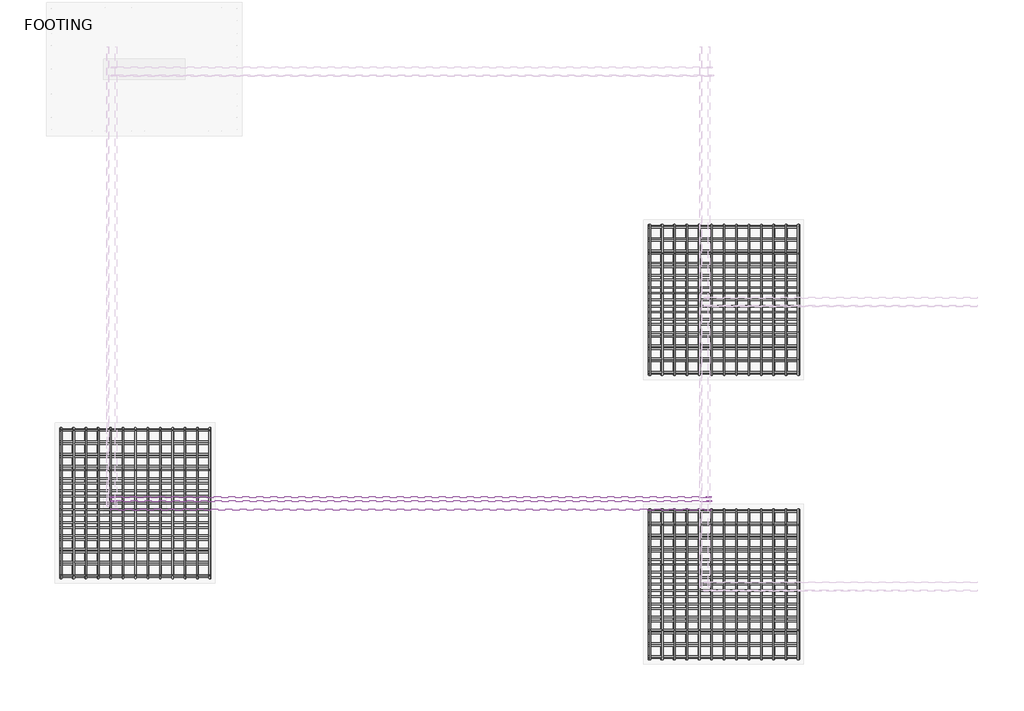
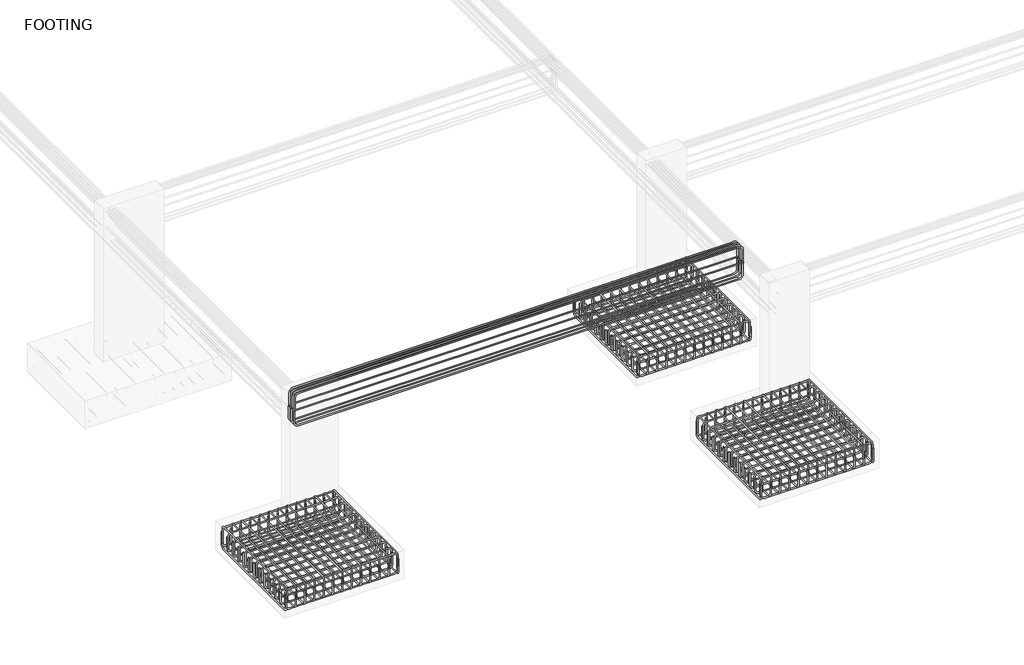
# One storey, part 2 of 12: 15 reinforcing bars.
"""IFC4 building model written with IfcOpenShell, lengths in millimetres."""

from ifc_helpers import new_model, si_unit, point, frame, origin, place, context, project, spatial, polyline, circle_curve, trimmed, segment, composite_curve, source, transform, mapped, element, save
from ifc_brep_helpers import swept_disk

model = new_model("IFC4")

# Units and contexts
model_context = context("Model", 3, world=origin())
ifc_project = project(units=[si_unit("LENGTHUNIT", "METRE", prefix="MILLI")], contexts=[model_context])

# Site, building, storey
site = spatial("IfcSite", under=ifc_project)
building = spatial("IfcBuilding", under=site)
storey = spatial("IfcBuildingStorey", under=building, Name="FOOTING", Elevation=-5638.8)

# Reinforcing bars
placement = place(None, origin())
reinforcing_bar_shape = source(origin(), model_context, "Body", "SolidModel", [
    swept_disk(composite_curve([segment(polyline([(-7583.1001665, -10857.5541655, -5788.8), (-7583.1001665, -10857.5541655, -5975.4)]), True, "CONTINUOUS"), segment(trimmed(circle_curve(frame((-7583.1001665, -10802.1041655, -5975.4), z_axis=(1.0, 0.0, 0.0), x_axis=(0.0, -55.44999999999891, 0.0)), 55.45), [point((-7583.1001665, -10857.5541655, -5975.4))], [point((-7583.1001665, -10802.1041655, -6030.85))], True, "CARTESIAN"), True, "CONTINUOUS"), segment(polyline([(-7583.1001665, -10802.1041655, -6030.85), (-7583.1001665, -9228.9041655, -6030.85)]), True, "CONTINUOUS"), segment(trimmed(circle_curve(frame((-7583.1001665, -9228.9041655, -5975.4), z_axis=(1.0, 0.0, 0.0), x_axis=(0.0, 0.0, -55.45000000000073)), 55.45), [point((-7583.1001665, -9228.9041655, -6030.85))], [point((-7583.1001665, -9173.4541655, -5975.4))], True, "CARTESIAN"), True, "CONTINUOUS"), segment(polyline([(-7583.1001665, -9173.4541655, -5975.4), (-7583.1001665, -9173.4541655, -5788.8)]), True, "CONTINUOUS")], self_intersect=False), 7.95),
])
element("IfcReinforcingBar", 1, at=placement, inside=storey, context=model_context, shape_type="MappedRepresentation", body=[
    mapped(reinforcing_bar_shape, transform((0.0, 0.0, 0.0), x_axis=(1.0, 0.0, 0.0), y_axis=(0.0, 1.0, 0.0), z_axis=(0.0, 0.0, 1.0))),
    mapped(reinforcing_bar_shape, transform((-140.3416667, 0.0, 0.0), x_axis=(1.0, 0.0, 0.0), y_axis=(0.0, 1.0, 0.0), z_axis=(0.0, 0.0, 1.0))),
    mapped(reinforcing_bar_shape, transform((-280.6833333, 0.0, 0.0), x_axis=(1.0, 0.0, 0.0), y_axis=(0.0, 1.0, 0.0), z_axis=(0.0, 0.0, 1.0))),
    mapped(reinforcing_bar_shape, transform((-421.025, 0.0, 0.0), x_axis=(1.0, 0.0, 0.0), y_axis=(0.0, 1.0, 0.0), z_axis=(0.0, 0.0, 1.0))),
    mapped(reinforcing_bar_shape, transform((-561.3666667, 0.0, 0.0), x_axis=(1.0, 0.0, 0.0), y_axis=(0.0, 1.0, 0.0), z_axis=(0.0, 0.0, 1.0))),
    mapped(reinforcing_bar_shape, transform((-701.7083333, 0.0, 0.0), x_axis=(1.0, 0.0, 0.0), y_axis=(0.0, 1.0, 0.0), z_axis=(0.0, 0.0, 1.0))),
    mapped(reinforcing_bar_shape, transform((-842.05, 0.0, 0.0), x_axis=(1.0, 0.0, 0.0), y_axis=(0.0, 1.0, 0.0), z_axis=(0.0, 0.0, 1.0))),
    mapped(reinforcing_bar_shape, transform((-982.3916667, 0.0, 0.0), x_axis=(1.0, 0.0, 0.0), y_axis=(0.0, 1.0, 0.0), z_axis=(0.0, 0.0, 1.0))),
    mapped(reinforcing_bar_shape, transform((-1122.7333333, 0.0, 0.0), x_axis=(1.0, 0.0, 0.0), y_axis=(0.0, 1.0, 0.0), z_axis=(0.0, 0.0, 1.0))),
    mapped(reinforcing_bar_shape, transform((-1263.075, 0.0, 0.0), x_axis=(1.0, 0.0, 0.0), y_axis=(0.0, 1.0, 0.0), z_axis=(0.0, 0.0, 1.0))),
    mapped(reinforcing_bar_shape, transform((-1403.4166667, 0.0, 0.0), x_axis=(1.0, 0.0, 0.0), y_axis=(0.0, 1.0, 0.0), z_axis=(0.0, 0.0, 1.0))),
    mapped(reinforcing_bar_shape, transform((-1543.7583333, 0.0, 0.0), x_axis=(1.0, 0.0, 0.0), y_axis=(0.0, 1.0, 0.0), z_axis=(0.0, 0.0, 1.0))),
    mapped(reinforcing_bar_shape, transform((-1684.1, 0.0, 0.0), x_axis=(1.0, 0.0, 0.0), y_axis=(0.0, 1.0, 0.0), z_axis=(0.0, 0.0, 1.0))),
])
reinforcing_bar_2_shape = source(origin(), model_context, "Body", "SolidModel", [
    swept_disk(composite_curve([segment(polyline([(-7592.2402006, -9171.8541655, -5888.8), (-7592.2402006, -9171.8541655, -5741.5)]), True, "CONTINUOUS"), segment(trimmed(circle_curve(frame((-7592.2402006, -9218.2041655, -5741.5), z_axis=(1.0, 0.0, 0.0), x_axis=(0.0, 46.349999999998545, 0.0)), 46.35), [point((-7592.2402006, -9171.8541655, -5741.5))], [point((-7592.2402006, -9218.2041655, -5695.15))], True, "CARTESIAN"), True, "CONTINUOUS"), segment(polyline([(-7592.2402006, -9218.2041655, -5695.15), (-7592.2402006, -10812.8041655, -5695.15)]), True, "CONTINUOUS"), segment(trimmed(circle_curve(frame((-7592.2402006, -10812.8041655, -5741.5), z_axis=(1.0, 0.0, 0.0), x_axis=(0.0, 0.0, 46.350000000000364)), 46.35), [point((-7592.2402006, -10812.8041655, -5695.15))], [point((-7592.2402006, -10859.1541655, -5741.5))], True, "CARTESIAN"), True, "CONTINUOUS"), segment(polyline([(-7592.2402006, -10859.1541655, -5741.5), (-7592.2402006, -10859.1541655, -5888.8)]), True, "CONTINUOUS")], self_intersect=False), 6.35),
])
element("IfcReinforcingBar", 2, at=placement, inside=storey, context=model_context, shape_type="MappedRepresentation", body=[
    mapped(reinforcing_bar_2_shape, transform((0.0, 0.0, 0.0), x_axis=(1.0, 0.0, 0.0), y_axis=(0.0, 1.0, 0.0), z_axis=(0.0, 0.0, 1.0))),
    mapped(reinforcing_bar_2_shape, transform((-138.4829293, 0.0, 0.0), x_axis=(1.0, 0.0, 0.0), y_axis=(0.0, 1.0, 0.0), z_axis=(0.0, 0.0, 1.0))),
    mapped(reinforcing_bar_2_shape, transform((-276.9658586, 0.0, 0.0), x_axis=(1.0, 0.0, 0.0), y_axis=(0.0, 1.0, 0.0), z_axis=(0.0, 0.0, 1.0))),
    mapped(reinforcing_bar_2_shape, transform((-415.4487879, 0.0, 0.0), x_axis=(1.0, 0.0, 0.0), y_axis=(0.0, 1.0, 0.0), z_axis=(0.0, 0.0, 1.0))),
    mapped(reinforcing_bar_2_shape, transform((-553.9317172, 0.0, 0.0), x_axis=(1.0, 0.0, 0.0), y_axis=(0.0, 1.0, 0.0), z_axis=(0.0, 0.0, 1.0))),
    mapped(reinforcing_bar_2_shape, transform((-692.4146465, 0.0, 0.0), x_axis=(1.0, 0.0, 0.0), y_axis=(0.0, 1.0, 0.0), z_axis=(0.0, 0.0, 1.0))),
    mapped(reinforcing_bar_2_shape, transform((-830.8975758, 0.0, 0.0), x_axis=(1.0, 0.0, 0.0), y_axis=(0.0, 1.0, 0.0), z_axis=(0.0, 0.0, 1.0))),
    mapped(reinforcing_bar_2_shape, transform((-969.3805051, 0.0, 0.0), x_axis=(1.0, 0.0, 0.0), y_axis=(0.0, 1.0, 0.0), z_axis=(0.0, 0.0, 1.0))),
    mapped(reinforcing_bar_2_shape, transform((-1107.8634344, 0.0, 0.0), x_axis=(1.0, 0.0, 0.0), y_axis=(0.0, 1.0, 0.0), z_axis=(0.0, 0.0, 1.0))),
    mapped(reinforcing_bar_2_shape, transform((-1246.3463637, 0.0, 0.0), x_axis=(1.0, 0.0, 0.0), y_axis=(0.0, 1.0, 0.0), z_axis=(0.0, 0.0, 1.0))),
    mapped(reinforcing_bar_2_shape, transform((-1384.8292929, 0.0, 0.0), x_axis=(1.0, 0.0, 0.0), y_axis=(0.0, 1.0, 0.0), z_axis=(0.0, 0.0, 1.0))),
    mapped(reinforcing_bar_2_shape, transform((-1523.3122222, 0.0, 0.0), x_axis=(1.0, 0.0, 0.0), y_axis=(0.0, 1.0, 0.0), z_axis=(0.0, 0.0, 1.0))),
    mapped(reinforcing_bar_2_shape, transform((-1661.7951515, 0.0, 0.0), x_axis=(1.0, 0.0, 0.0), y_axis=(0.0, 1.0, 0.0), z_axis=(0.0, 0.0, 1.0))),
])
reinforcing_bar_3_shape = source(origin(), model_context, "Body", "SolidModel", [
    swept_disk(composite_curve([segment(polyline([(-9267.2001665, -10840.5041655, -5773.0), (-9267.2001665, -10840.5041655, -5959.6)]), True, "CONTINUOUS"), segment(trimmed(circle_curve(frame((-9211.7501665, -10840.5041655, -5959.6), z_axis=(0.0, -1.0, 0.0), x_axis=(-55.45000000000073, 0.0, 0.0)), 55.45), [point((-9267.2001665, -10840.5041655, -5959.6))], [point((-9211.7501665, -10840.5041655, -6015.05))], True, "CARTESIAN"), True, "CONTINUOUS"), segment(polyline([(-9211.7501665, -10840.5041655, -6015.05), (-7638.5501665, -10840.5041655, -6015.05)]), True, "CONTINUOUS"), segment(trimmed(circle_curve(frame((-7638.5501665, -10840.5041655, -5959.6), z_axis=(0.0, -1.0, 0.0), x_axis=(0.0, 0.0, -55.44999999999982)), 55.45), [point((-7638.5501665, -10840.5041655, -6015.05))], [point((-7583.1001665, -10840.5041655, -5959.6))], True, "CARTESIAN"), True, "CONTINUOUS"), segment(polyline([(-7583.1001665, -10840.5041655, -5959.6), (-7583.1001665, -10840.5041655, -5773.0)]), True, "CONTINUOUS")], self_intersect=False), 7.95),
])
element("IfcReinforcingBar", 3, at=placement, inside=storey, context=model_context, shape_type="MappedRepresentation", body=[
    mapped(reinforcing_bar_3_shape, transform((0.0, 0.0, 0.0), x_axis=(1.0, 0.0, 0.0), y_axis=(0.0, 1.0, 0.0), z_axis=(0.0, 0.0, 1.0))),
    mapped(reinforcing_bar_3_shape, transform((0.0, 137.7402087, 0.0), x_axis=(1.0, 0.0, 0.0), y_axis=(0.0, 1.0, 0.0), z_axis=(0.0, 0.0, 1.0))),
    mapped(reinforcing_bar_3_shape, transform((0.0, 275.4804175, 0.0), x_axis=(1.0, 0.0, 0.0), y_axis=(0.0, 1.0, 0.0), z_axis=(0.0, 0.0, 1.0))),
    mapped(reinforcing_bar_3_shape, transform((0.0, 413.2206262, 0.0), x_axis=(1.0, 0.0, 0.0), y_axis=(0.0, 1.0, 0.0), z_axis=(0.0, 0.0, 1.0))),
    mapped(reinforcing_bar_3_shape, transform((0.0, 550.960835, 0.0), x_axis=(1.0, 0.0, 0.0), y_axis=(0.0, 1.0, 0.0), z_axis=(0.0, 0.0, 1.0))),
    mapped(reinforcing_bar_3_shape, transform((0.0, 688.7010437, 0.0), x_axis=(1.0, 0.0, 0.0), y_axis=(0.0, 1.0, 0.0), z_axis=(0.0, 0.0, 1.0))),
    mapped(reinforcing_bar_3_shape, transform((0.0, 826.4412525, 0.0), x_axis=(1.0, 0.0, 0.0), y_axis=(0.0, 1.0, 0.0), z_axis=(0.0, 0.0, 1.0))),
    mapped(reinforcing_bar_3_shape, transform((0.0, 964.1814612, 0.0), x_axis=(1.0, 0.0, 0.0), y_axis=(0.0, 1.0, 0.0), z_axis=(0.0, 0.0, 1.0))),
    mapped(reinforcing_bar_3_shape, transform((0.0, 1101.92167, 0.0), x_axis=(1.0, 0.0, 0.0), y_axis=(0.0, 1.0, 0.0), z_axis=(0.0, 0.0, 1.0))),
    mapped(reinforcing_bar_3_shape, transform((0.0, 1239.6618787, 0.0), x_axis=(1.0, 0.0, 0.0), y_axis=(0.0, 1.0, 0.0), z_axis=(0.0, 0.0, 1.0))),
    mapped(reinforcing_bar_3_shape, transform((0.0, 1377.4020875, 0.0), x_axis=(1.0, 0.0, 0.0), y_axis=(0.0, 1.0, 0.0), z_axis=(0.0, 0.0, 1.0))),
    mapped(reinforcing_bar_3_shape, transform((0.0, 1515.1422962, 0.0), x_axis=(1.0, 0.0, 0.0), y_axis=(0.0, 1.0, 0.0), z_axis=(0.0, 0.0, 1.0))),
    mapped(reinforcing_bar_3_shape, transform((0.0, 1652.882505, 0.0), x_axis=(1.0, 0.0, 0.0), y_axis=(0.0, 1.0, 0.0), z_axis=(0.0, 0.0, 1.0))),
])
reinforcing_bar_4_shape = source(origin(), model_context, "Body", "SolidModel", [
    swept_disk(composite_curve([segment(polyline([(-9267.2001665, -9197.8399866, -5950.85), (-9267.2001665, -9197.8399866, -5764.25)]), True, "CONTINUOUS"), segment(trimmed(circle_curve(frame((-9211.7501665, -9197.8399866, -5764.25), z_axis=(0.0, 1.0, 0.0), x_axis=(-55.45000000000073, 0.0, 0.0)), 55.45), [point((-9267.2001665, -9197.8399866, -5764.25))], [point((-9211.7501665, -9197.8399866, -5708.8))], True, "CARTESIAN"), True, "CONTINUOUS"), segment(polyline([(-9211.7501665, -9197.8399866, -5708.8), (-7638.5501665, -9197.8399866, -5708.8)]), True, "CONTINUOUS"), segment(trimmed(circle_curve(frame((-7638.5501665, -9197.8399866, -5764.25), z_axis=(0.0, 1.0, 0.0), x_axis=(0.0, 0.0, 55.44999999999982)), 55.45), [point((-7638.5501665, -9197.8399866, -5708.8))], [point((-7583.1001665, -9197.8399866, -5764.25))], True, "CARTESIAN"), True, "CONTINUOUS"), segment(polyline([(-7583.1001665, -9197.8399866, -5764.25), (-7583.1001665, -9197.8399866, -5950.85)]), True, "CONTINUOUS")], self_intersect=False), 7.95),
])
element("IfcReinforcingBar", 4, at=placement, inside=storey, context=model_context, shape_type="MappedRepresentation", body=[
    mapped(reinforcing_bar_4_shape, transform((0.0, 0.0, 0.0), x_axis=(1.0, 0.0, 0.0), y_axis=(0.0, 1.0, 0.0), z_axis=(0.0, 0.0, 1.0))),
    mapped(reinforcing_bar_4_shape, transform((0.0, -148.1882348, 0.0), x_axis=(1.0, 0.0, 0.0), y_axis=(0.0, 1.0, 0.0), z_axis=(0.0, 0.0, 1.0))),
    mapped(reinforcing_bar_4_shape, transform((0.0, -296.3764695, 0.0), x_axis=(1.0, 0.0, 0.0), y_axis=(0.0, 1.0, 0.0), z_axis=(0.0, 0.0, 1.0))),
    mapped(reinforcing_bar_4_shape, transform((0.0, -444.5647043, 0.0), x_axis=(1.0, 0.0, 0.0), y_axis=(0.0, 1.0, 0.0), z_axis=(0.0, 0.0, 1.0))),
    mapped(reinforcing_bar_4_shape, transform((0.0, -592.7529391, 0.0), x_axis=(1.0, 0.0, 0.0), y_axis=(0.0, 1.0, 0.0), z_axis=(0.0, 0.0, 1.0))),
    mapped(reinforcing_bar_4_shape, transform((0.0, -740.9411738, 0.0), x_axis=(1.0, 0.0, 0.0), y_axis=(0.0, 1.0, 0.0), z_axis=(0.0, 0.0, 1.0))),
    mapped(reinforcing_bar_4_shape, transform((0.0, -889.1294086, 0.0), x_axis=(1.0, 0.0, 0.0), y_axis=(0.0, 1.0, 0.0), z_axis=(0.0, 0.0, 1.0))),
    mapped(reinforcing_bar_4_shape, transform((0.0, -1037.3176434, 0.0), x_axis=(1.0, 0.0, 0.0), y_axis=(0.0, 1.0, 0.0), z_axis=(0.0, 0.0, 1.0))),
    mapped(reinforcing_bar_4_shape, transform((0.0, -1185.5058782, 0.0), x_axis=(1.0, 0.0, 0.0), y_axis=(0.0, 1.0, 0.0), z_axis=(0.0, 0.0, 1.0))),
    mapped(reinforcing_bar_4_shape, transform((0.0, -1333.6941129, 0.0), x_axis=(1.0, 0.0, 0.0), y_axis=(0.0, 1.0, 0.0), z_axis=(0.0, 0.0, 1.0))),
    mapped(reinforcing_bar_4_shape, transform((0.0, -1481.8823477, 0.0), x_axis=(1.0, 0.0, 0.0), y_axis=(0.0, 1.0, 0.0), z_axis=(0.0, 0.0, 1.0))),
    mapped(reinforcing_bar_4_shape, transform((0.0, -1630.0705825, 0.0), x_axis=(1.0, 0.0, 0.0), y_axis=(0.0, 1.0, 0.0), z_axis=(0.0, 0.0, 1.0))),
])
reinforcing_bar_5_shape = source(origin(), model_context, "Body", "SolidModel", [
    swept_disk(composite_curve([segment(polyline([(-7583.1001665, -14057.9541655, -5788.8), (-7583.1001665, -14057.9541655, -5975.4)]), True, "CONTINUOUS"), segment(trimmed(circle_curve(frame((-7583.1001665, -14002.5041655, -5975.4), z_axis=(1.0, 0.0, 0.0), x_axis=(0.0, -55.44999999999891, 0.0)), 55.45), [point((-7583.1001665, -14057.9541655, -5975.4))], [point((-7583.1001665, -14002.5041655, -6030.85))], True, "CARTESIAN"), True, "CONTINUOUS"), segment(polyline([(-7583.1001665, -14002.5041655, -6030.85), (-7583.1001665, -12429.3041655, -6030.85)]), True, "CONTINUOUS"), segment(trimmed(circle_curve(frame((-7583.1001665, -12429.3041655, -5975.4), z_axis=(1.0, 0.0, 0.0), x_axis=(0.0, 0.0, -55.45000000000073)), 55.45), [point((-7583.1001665, -12429.3041655, -6030.85))], [point((-7583.1001665, -12373.8541655, -5975.4))], True, "CARTESIAN"), True, "CONTINUOUS"), segment(polyline([(-7583.1001665, -12373.8541655, -5975.4), (-7583.1001665, -12373.8541655, -5788.8)]), True, "CONTINUOUS")], self_intersect=False), 7.95),
])
element("IfcReinforcingBar", 5, at=placement, inside=storey, context=model_context, shape_type="MappedRepresentation", body=[
    mapped(reinforcing_bar_5_shape, transform((0.0, 0.0, 0.0), x_axis=(1.0, 0.0, 0.0), y_axis=(0.0, 1.0, 0.0), z_axis=(0.0, 0.0, 1.0))),
    mapped(reinforcing_bar_5_shape, transform((-140.3416667, 0.0, 0.0), x_axis=(1.0, 0.0, 0.0), y_axis=(0.0, 1.0, 0.0), z_axis=(0.0, 0.0, 1.0))),
    mapped(reinforcing_bar_5_shape, transform((-280.6833333, 0.0, 0.0), x_axis=(1.0, 0.0, 0.0), y_axis=(0.0, 1.0, 0.0), z_axis=(0.0, 0.0, 1.0))),
    mapped(reinforcing_bar_5_shape, transform((-421.025, 0.0, 0.0), x_axis=(1.0, 0.0, 0.0), y_axis=(0.0, 1.0, 0.0), z_axis=(0.0, 0.0, 1.0))),
    mapped(reinforcing_bar_5_shape, transform((-561.3666667, 0.0, 0.0), x_axis=(1.0, 0.0, 0.0), y_axis=(0.0, 1.0, 0.0), z_axis=(0.0, 0.0, 1.0))),
    mapped(reinforcing_bar_5_shape, transform((-701.7083333, 0.0, 0.0), x_axis=(1.0, 0.0, 0.0), y_axis=(0.0, 1.0, 0.0), z_axis=(0.0, 0.0, 1.0))),
    mapped(reinforcing_bar_5_shape, transform((-842.05, 0.0, 0.0), x_axis=(1.0, 0.0, 0.0), y_axis=(0.0, 1.0, 0.0), z_axis=(0.0, 0.0, 1.0))),
    mapped(reinforcing_bar_5_shape, transform((-982.3916667, 0.0, 0.0), x_axis=(1.0, 0.0, 0.0), y_axis=(0.0, 1.0, 0.0), z_axis=(0.0, 0.0, 1.0))),
    mapped(reinforcing_bar_5_shape, transform((-1122.7333333, 0.0, 0.0), x_axis=(1.0, 0.0, 0.0), y_axis=(0.0, 1.0, 0.0), z_axis=(0.0, 0.0, 1.0))),
    mapped(reinforcing_bar_5_shape, transform((-1263.075, 0.0, 0.0), x_axis=(1.0, 0.0, 0.0), y_axis=(0.0, 1.0, 0.0), z_axis=(0.0, 0.0, 1.0))),
    mapped(reinforcing_bar_5_shape, transform((-1403.4166667, 0.0, 0.0), x_axis=(1.0, 0.0, 0.0), y_axis=(0.0, 1.0, 0.0), z_axis=(0.0, 0.0, 1.0))),
    mapped(reinforcing_bar_5_shape, transform((-1543.7583333, 0.0, 0.0), x_axis=(1.0, 0.0, 0.0), y_axis=(0.0, 1.0, 0.0), z_axis=(0.0, 0.0, 1.0))),
    mapped(reinforcing_bar_5_shape, transform((-1684.1, 0.0, 0.0), x_axis=(1.0, 0.0, 0.0), y_axis=(0.0, 1.0, 0.0), z_axis=(0.0, 0.0, 1.0))),
])
reinforcing_bar_6_shape = source(origin(), model_context, "Body", "SolidModel", [
    swept_disk(composite_curve([segment(polyline([(-7592.2402006, -12372.2541655, -5888.8), (-7592.2402006, -12372.2541655, -5741.5)]), True, "CONTINUOUS"), segment(trimmed(circle_curve(frame((-7592.2402006, -12418.6041655, -5741.5), z_axis=(1.0, 0.0, 0.0), x_axis=(0.0, 46.350000000000364, 0.0)), 46.35), [point((-7592.2402006, -12372.2541655, -5741.5))], [point((-7592.2402006, -12418.6041655, -5695.15))], True, "CARTESIAN"), True, "CONTINUOUS"), segment(polyline([(-7592.2402006, -12418.6041655, -5695.15), (-7592.2402006, -14013.2041655, -5695.15)]), True, "CONTINUOUS"), segment(trimmed(circle_curve(frame((-7592.2402006, -14013.2041655, -5741.5), z_axis=(1.0, 0.0, 0.0), x_axis=(0.0, 0.0, 46.350000000000364)), 46.35), [point((-7592.2402006, -14013.2041655, -5695.15))], [point((-7592.2402006, -14059.5541655, -5741.5))], True, "CARTESIAN"), True, "CONTINUOUS"), segment(polyline([(-7592.2402006, -14059.5541655, -5741.5), (-7592.2402006, -14059.5541655, -5888.8)]), True, "CONTINUOUS")], self_intersect=False), 6.35),
])
element("IfcReinforcingBar", 6, at=placement, inside=storey, context=model_context, shape_type="MappedRepresentation", body=[
    mapped(reinforcing_bar_6_shape, transform((0.0, 0.0, 0.0), x_axis=(1.0, 0.0, 0.0), y_axis=(0.0, 1.0, 0.0), z_axis=(0.0, 0.0, 1.0))),
    mapped(reinforcing_bar_6_shape, transform((-138.4829293, 0.0, 0.0), x_axis=(1.0, 0.0, 0.0), y_axis=(0.0, 1.0, 0.0), z_axis=(0.0, 0.0, 1.0))),
    mapped(reinforcing_bar_6_shape, transform((-276.9658586, 0.0, 0.0), x_axis=(1.0, 0.0, 0.0), y_axis=(0.0, 1.0, 0.0), z_axis=(0.0, 0.0, 1.0))),
    mapped(reinforcing_bar_6_shape, transform((-415.4487879, 0.0, 0.0), x_axis=(1.0, 0.0, 0.0), y_axis=(0.0, 1.0, 0.0), z_axis=(0.0, 0.0, 1.0))),
    mapped(reinforcing_bar_6_shape, transform((-553.9317172, 0.0, 0.0), x_axis=(1.0, 0.0, 0.0), y_axis=(0.0, 1.0, 0.0), z_axis=(0.0, 0.0, 1.0))),
    mapped(reinforcing_bar_6_shape, transform((-692.4146465, 0.0, 0.0), x_axis=(1.0, 0.0, 0.0), y_axis=(0.0, 1.0, 0.0), z_axis=(0.0, 0.0, 1.0))),
    mapped(reinforcing_bar_6_shape, transform((-830.8975758, 0.0, 0.0), x_axis=(1.0, 0.0, 0.0), y_axis=(0.0, 1.0, 0.0), z_axis=(0.0, 0.0, 1.0))),
    mapped(reinforcing_bar_6_shape, transform((-969.3805051, 0.0, 0.0), x_axis=(1.0, 0.0, 0.0), y_axis=(0.0, 1.0, 0.0), z_axis=(0.0, 0.0, 1.0))),
    mapped(reinforcing_bar_6_shape, transform((-1107.8634344, 0.0, 0.0), x_axis=(1.0, 0.0, 0.0), y_axis=(0.0, 1.0, 0.0), z_axis=(0.0, 0.0, 1.0))),
    mapped(reinforcing_bar_6_shape, transform((-1246.3463637, 0.0, 0.0), x_axis=(1.0, 0.0, 0.0), y_axis=(0.0, 1.0, 0.0), z_axis=(0.0, 0.0, 1.0))),
    mapped(reinforcing_bar_6_shape, transform((-1384.8292929, 0.0, 0.0), x_axis=(1.0, 0.0, 0.0), y_axis=(0.0, 1.0, 0.0), z_axis=(0.0, 0.0, 1.0))),
    mapped(reinforcing_bar_6_shape, transform((-1523.3122222, 0.0, 0.0), x_axis=(1.0, 0.0, 0.0), y_axis=(0.0, 1.0, 0.0), z_axis=(0.0, 0.0, 1.0))),
    mapped(reinforcing_bar_6_shape, transform((-1661.7951515, 0.0, 0.0), x_axis=(1.0, 0.0, 0.0), y_axis=(0.0, 1.0, 0.0), z_axis=(0.0, 0.0, 1.0))),
])
reinforcing_bar_7_shape = source(origin(), model_context, "Body", "SolidModel", [
    swept_disk(composite_curve([segment(polyline([(-9267.2001665, -14040.9041655, -5773.0), (-9267.2001665, -14040.9041655, -5959.6)]), True, "CONTINUOUS"), segment(trimmed(circle_curve(frame((-9211.7501665, -14040.9041655, -5959.6), z_axis=(0.0, -1.0, 0.0), x_axis=(-55.45000000000073, 0.0, 0.0)), 55.45), [point((-9267.2001665, -14040.9041655, -5959.6))], [point((-9211.7501665, -14040.9041655, -6015.05))], True, "CARTESIAN"), True, "CONTINUOUS"), segment(polyline([(-9211.7501665, -14040.9041655, -6015.05), (-7638.5501665, -14040.9041655, -6015.05)]), True, "CONTINUOUS"), segment(trimmed(circle_curve(frame((-7638.5501665, -14040.9041655, -5959.6), z_axis=(0.0, -1.0, 0.0), x_axis=(0.0, 0.0, -55.44999999999982)), 55.45), [point((-7638.5501665, -14040.9041655, -6015.05))], [point((-7583.1001665, -14040.9041655, -5959.6))], True, "CARTESIAN"), True, "CONTINUOUS"), segment(polyline([(-7583.1001665, -14040.9041655, -5959.6), (-7583.1001665, -14040.9041655, -5773.0)]), True, "CONTINUOUS")], self_intersect=False), 7.95),
])
element("IfcReinforcingBar", 7, at=placement, inside=storey, context=model_context, shape_type="MappedRepresentation", body=[
    mapped(reinforcing_bar_7_shape, transform((0.0, 0.0, 0.0), x_axis=(1.0, 0.0, 0.0), y_axis=(0.0, 1.0, 0.0), z_axis=(0.0, 0.0, 1.0))),
    mapped(reinforcing_bar_7_shape, transform((0.0, 137.7402087, 0.0), x_axis=(1.0, 0.0, 0.0), y_axis=(0.0, 1.0, 0.0), z_axis=(0.0, 0.0, 1.0))),
    mapped(reinforcing_bar_7_shape, transform((0.0, 275.4804175, 0.0), x_axis=(1.0, 0.0, 0.0), y_axis=(0.0, 1.0, 0.0), z_axis=(0.0, 0.0, 1.0))),
    mapped(reinforcing_bar_7_shape, transform((0.0, 413.2206262, 0.0), x_axis=(1.0, 0.0, 0.0), y_axis=(0.0, 1.0, 0.0), z_axis=(0.0, 0.0, 1.0))),
    mapped(reinforcing_bar_7_shape, transform((0.0, 550.960835, 0.0), x_axis=(1.0, 0.0, 0.0), y_axis=(0.0, 1.0, 0.0), z_axis=(0.0, 0.0, 1.0))),
    mapped(reinforcing_bar_7_shape, transform((0.0, 688.7010437, 0.0), x_axis=(1.0, 0.0, 0.0), y_axis=(0.0, 1.0, 0.0), z_axis=(0.0, 0.0, 1.0))),
    mapped(reinforcing_bar_7_shape, transform((0.0, 826.4412525, 0.0), x_axis=(1.0, 0.0, 0.0), y_axis=(0.0, 1.0, 0.0), z_axis=(0.0, 0.0, 1.0))),
    mapped(reinforcing_bar_7_shape, transform((0.0, 964.1814612, 0.0), x_axis=(1.0, 0.0, 0.0), y_axis=(0.0, 1.0, 0.0), z_axis=(0.0, 0.0, 1.0))),
    mapped(reinforcing_bar_7_shape, transform((0.0, 1101.92167, 0.0), x_axis=(1.0, 0.0, 0.0), y_axis=(0.0, 1.0, 0.0), z_axis=(0.0, 0.0, 1.0))),
    mapped(reinforcing_bar_7_shape, transform((0.0, 1239.6618787, 0.0), x_axis=(1.0, 0.0, 0.0), y_axis=(0.0, 1.0, 0.0), z_axis=(0.0, 0.0, 1.0))),
    mapped(reinforcing_bar_7_shape, transform((0.0, 1377.4020875, 0.0), x_axis=(1.0, 0.0, 0.0), y_axis=(0.0, 1.0, 0.0), z_axis=(0.0, 0.0, 1.0))),
    mapped(reinforcing_bar_7_shape, transform((0.0, 1515.1422962, 0.0), x_axis=(1.0, 0.0, 0.0), y_axis=(0.0, 1.0, 0.0), z_axis=(0.0, 0.0, 1.0))),
    mapped(reinforcing_bar_7_shape, transform((0.0, 1652.882505, 0.0), x_axis=(1.0, 0.0, 0.0), y_axis=(0.0, 1.0, 0.0), z_axis=(0.0, 0.0, 1.0))),
])
reinforcing_bar_8_shape = source(origin(), model_context, "Body", "SolidModel", [
    swept_disk(composite_curve([segment(polyline([(-9267.2001665, -12398.2399866, -5950.85), (-9267.2001665, -12398.2399866, -5764.25)]), True, "CONTINUOUS"), segment(trimmed(circle_curve(frame((-9211.7501665, -12398.2399866, -5764.25), z_axis=(0.0, 1.0, 0.0), x_axis=(-55.45000000000073, 0.0, 0.0)), 55.45), [point((-9267.2001665, -12398.2399866, -5764.25))], [point((-9211.7501665, -12398.2399866, -5708.8))], True, "CARTESIAN"), True, "CONTINUOUS"), segment(polyline([(-9211.7501665, -12398.2399866, -5708.8), (-7638.5501665, -12398.2399866, -5708.8)]), True, "CONTINUOUS"), segment(trimmed(circle_curve(frame((-7638.5501665, -12398.2399866, -5764.25), z_axis=(0.0, 1.0, 0.0), x_axis=(0.0, 0.0, 55.44999999999982)), 55.45), [point((-7638.5501665, -12398.2399866, -5708.8))], [point((-7583.1001665, -12398.2399866, -5764.25))], True, "CARTESIAN"), True, "CONTINUOUS"), segment(polyline([(-7583.1001665, -12398.2399866, -5764.25), (-7583.1001665, -12398.2399866, -5950.85)]), True, "CONTINUOUS")], self_intersect=False), 7.95),
])
element("IfcReinforcingBar", 8, at=placement, inside=storey, context=model_context, shape_type="MappedRepresentation", body=[
    mapped(reinforcing_bar_8_shape, transform((0.0, 0.0, 0.0), x_axis=(1.0, 0.0, 0.0), y_axis=(0.0, 1.0, 0.0), z_axis=(0.0, 0.0, 1.0))),
    mapped(reinforcing_bar_8_shape, transform((0.0, -148.1882348, 0.0), x_axis=(1.0, 0.0, 0.0), y_axis=(0.0, 1.0, 0.0), z_axis=(0.0, 0.0, 1.0))),
    mapped(reinforcing_bar_8_shape, transform((0.0, -296.3764695, 0.0), x_axis=(1.0, 0.0, 0.0), y_axis=(0.0, 1.0, 0.0), z_axis=(0.0, 0.0, 1.0))),
    mapped(reinforcing_bar_8_shape, transform((0.0, -444.5647043, 0.0), x_axis=(1.0, 0.0, 0.0), y_axis=(0.0, 1.0, 0.0), z_axis=(0.0, 0.0, 1.0))),
    mapped(reinforcing_bar_8_shape, transform((0.0, -592.7529391, 0.0), x_axis=(1.0, 0.0, 0.0), y_axis=(0.0, 1.0, 0.0), z_axis=(0.0, 0.0, 1.0))),
    mapped(reinforcing_bar_8_shape, transform((0.0, -740.9411738, 0.0), x_axis=(1.0, 0.0, 0.0), y_axis=(0.0, 1.0, 0.0), z_axis=(0.0, 0.0, 1.0))),
    mapped(reinforcing_bar_8_shape, transform((0.0, -889.1294086, 0.0), x_axis=(1.0, 0.0, 0.0), y_axis=(0.0, 1.0, 0.0), z_axis=(0.0, 0.0, 1.0))),
    mapped(reinforcing_bar_8_shape, transform((0.0, -1037.3176434, 0.0), x_axis=(1.0, 0.0, 0.0), y_axis=(0.0, 1.0, 0.0), z_axis=(0.0, 0.0, 1.0))),
    mapped(reinforcing_bar_8_shape, transform((0.0, -1185.5058782, 0.0), x_axis=(1.0, 0.0, 0.0), y_axis=(0.0, 1.0, 0.0), z_axis=(0.0, 0.0, 1.0))),
    mapped(reinforcing_bar_8_shape, transform((0.0, -1333.6941129, 0.0), x_axis=(1.0, 0.0, 0.0), y_axis=(0.0, 1.0, 0.0), z_axis=(0.0, 0.0, 1.0))),
    mapped(reinforcing_bar_8_shape, transform((0.0, -1481.8823477, 0.0), x_axis=(1.0, 0.0, 0.0), y_axis=(0.0, 1.0, 0.0), z_axis=(0.0, 0.0, 1.0))),
    mapped(reinforcing_bar_8_shape, transform((0.0, -1630.0705825, 0.0), x_axis=(1.0, 0.0, 0.0), y_axis=(0.0, 1.0, 0.0), z_axis=(0.0, 0.0, 1.0))),
])
reinforcing_bar_9_shape = source(origin(), model_context, "Body", "SolidModel", [
    swept_disk(composite_curve([segment(polyline([(-14199.8001665, -13143.5541655, -5788.8), (-14199.8001665, -13143.5541655, -5975.4)]), True, "CONTINUOUS"), segment(trimmed(circle_curve(frame((-14199.8001665, -13088.1041655, -5975.4), z_axis=(1.0, 0.0, 0.0), x_axis=(0.0, -55.44999999999891, 0.0)), 55.45), [point((-14199.8001665, -13143.5541655, -5975.4))], [point((-14199.8001665, -13088.1041655, -6030.85))], True, "CARTESIAN"), True, "CONTINUOUS"), segment(polyline([(-14199.8001665, -13088.1041655, -6030.85), (-14199.8001665, -11514.9041655, -6030.85)]), True, "CONTINUOUS"), segment(trimmed(circle_curve(frame((-14199.8001665, -11514.9041655, -5975.4), z_axis=(1.0, 0.0, 0.0), x_axis=(0.0, 0.0, -55.45000000000073)), 55.45), [point((-14199.8001665, -11514.9041655, -6030.85))], [point((-14199.8001665, -11459.4541655, -5975.4))], True, "CARTESIAN"), True, "CONTINUOUS"), segment(polyline([(-14199.8001665, -11459.4541655, -5975.4), (-14199.8001665, -11459.4541655, -5788.8)]), True, "CONTINUOUS")], self_intersect=False), 7.95),
])
element("IfcReinforcingBar", 9, at=placement, inside=storey, context=model_context, shape_type="MappedRepresentation", body=[
    mapped(reinforcing_bar_9_shape, transform((0.0, 0.0, 0.0), x_axis=(1.0, 0.0, 0.0), y_axis=(0.0, 1.0, 0.0), z_axis=(0.0, 0.0, 1.0))),
    mapped(reinforcing_bar_9_shape, transform((-140.3416667, 0.0, 0.0), x_axis=(1.0, 0.0, 0.0), y_axis=(0.0, 1.0, 0.0), z_axis=(0.0, 0.0, 1.0))),
    mapped(reinforcing_bar_9_shape, transform((-280.6833333, 0.0, 0.0), x_axis=(1.0, 0.0, 0.0), y_axis=(0.0, 1.0, 0.0), z_axis=(0.0, 0.0, 1.0))),
    mapped(reinforcing_bar_9_shape, transform((-421.025, 0.0, 0.0), x_axis=(1.0, 0.0, 0.0), y_axis=(0.0, 1.0, 0.0), z_axis=(0.0, 0.0, 1.0))),
    mapped(reinforcing_bar_9_shape, transform((-561.3666667, 0.0, 0.0), x_axis=(1.0, 0.0, 0.0), y_axis=(0.0, 1.0, 0.0), z_axis=(0.0, 0.0, 1.0))),
    mapped(reinforcing_bar_9_shape, transform((-701.7083333, 0.0, 0.0), x_axis=(1.0, 0.0, 0.0), y_axis=(0.0, 1.0, 0.0), z_axis=(0.0, 0.0, 1.0))),
    mapped(reinforcing_bar_9_shape, transform((-842.05, 0.0, 0.0), x_axis=(1.0, 0.0, 0.0), y_axis=(0.0, 1.0, 0.0), z_axis=(0.0, 0.0, 1.0))),
    mapped(reinforcing_bar_9_shape, transform((-982.3916667, 0.0, 0.0), x_axis=(1.0, 0.0, 0.0), y_axis=(0.0, 1.0, 0.0), z_axis=(0.0, 0.0, 1.0))),
    mapped(reinforcing_bar_9_shape, transform((-1122.7333333, 0.0, 0.0), x_axis=(1.0, 0.0, 0.0), y_axis=(0.0, 1.0, 0.0), z_axis=(0.0, 0.0, 1.0))),
    mapped(reinforcing_bar_9_shape, transform((-1263.075, 0.0, 0.0), x_axis=(1.0, 0.0, 0.0), y_axis=(0.0, 1.0, 0.0), z_axis=(0.0, 0.0, 1.0))),
    mapped(reinforcing_bar_9_shape, transform((-1403.4166667, 0.0, 0.0), x_axis=(1.0, 0.0, 0.0), y_axis=(0.0, 1.0, 0.0), z_axis=(0.0, 0.0, 1.0))),
    mapped(reinforcing_bar_9_shape, transform((-1543.7583333, 0.0, 0.0), x_axis=(1.0, 0.0, 0.0), y_axis=(0.0, 1.0, 0.0), z_axis=(0.0, 0.0, 1.0))),
    mapped(reinforcing_bar_9_shape, transform((-1684.1, 0.0, 0.0), x_axis=(1.0, 0.0, 0.0), y_axis=(0.0, 1.0, 0.0), z_axis=(0.0, 0.0, 1.0))),
])
reinforcing_bar_10_shape = source(origin(), model_context, "Body", "SolidModel", [
    swept_disk(composite_curve([segment(polyline([(-14208.9402006, -11457.8541655, -5888.8), (-14208.9402006, -11457.8541655, -5741.5)]), True, "CONTINUOUS"), segment(trimmed(circle_curve(frame((-14208.9402006, -11504.2041655, -5741.5), z_axis=(1.0, 0.0, 0.0), x_axis=(0.0, 46.349999999998545, 0.0)), 46.35), [point((-14208.9402006, -11457.8541655, -5741.5))], [point((-14208.9402006, -11504.2041655, -5695.15))], True, "CARTESIAN"), True, "CONTINUOUS"), segment(polyline([(-14208.9402006, -11504.2041655, -5695.15), (-14208.9402006, -13098.8041655, -5695.15)]), True, "CONTINUOUS"), segment(trimmed(circle_curve(frame((-14208.9402006, -13098.8041655, -5741.5), z_axis=(1.0, 0.0, 0.0), x_axis=(0.0, 0.0, 46.350000000000364)), 46.35), [point((-14208.9402006, -13098.8041655, -5695.15))], [point((-14208.9402006, -13145.1541655, -5741.5))], True, "CARTESIAN"), True, "CONTINUOUS"), segment(polyline([(-14208.9402006, -13145.1541655, -5741.5), (-14208.9402006, -13145.1541655, -5888.8)]), True, "CONTINUOUS")], self_intersect=False), 6.35),
])
element("IfcReinforcingBar", 10, at=placement, inside=storey, context=model_context, shape_type="MappedRepresentation", body=[
    mapped(reinforcing_bar_10_shape, transform((0.0, 0.0, 0.0), x_axis=(1.0, 0.0, 0.0), y_axis=(0.0, 1.0, 0.0), z_axis=(0.0, 0.0, 1.0))),
    mapped(reinforcing_bar_10_shape, transform((-138.4829293, 0.0, 0.0), x_axis=(1.0, 0.0, 0.0), y_axis=(0.0, 1.0, 0.0), z_axis=(0.0, 0.0, 1.0))),
    mapped(reinforcing_bar_10_shape, transform((-276.9658586, 0.0, 0.0), x_axis=(1.0, 0.0, 0.0), y_axis=(0.0, 1.0, 0.0), z_axis=(0.0, 0.0, 1.0))),
    mapped(reinforcing_bar_10_shape, transform((-415.4487879, 0.0, 0.0), x_axis=(1.0, 0.0, 0.0), y_axis=(0.0, 1.0, 0.0), z_axis=(0.0, 0.0, 1.0))),
    mapped(reinforcing_bar_10_shape, transform((-553.9317172, 0.0, 0.0), x_axis=(1.0, 0.0, 0.0), y_axis=(0.0, 1.0, 0.0), z_axis=(0.0, 0.0, 1.0))),
    mapped(reinforcing_bar_10_shape, transform((-692.4146465, 0.0, 0.0), x_axis=(1.0, 0.0, 0.0), y_axis=(0.0, 1.0, 0.0), z_axis=(0.0, 0.0, 1.0))),
    mapped(reinforcing_bar_10_shape, transform((-830.8975758, 0.0, 0.0), x_axis=(1.0, 0.0, 0.0), y_axis=(0.0, 1.0, 0.0), z_axis=(0.0, 0.0, 1.0))),
    mapped(reinforcing_bar_10_shape, transform((-969.3805051, 0.0, 0.0), x_axis=(1.0, 0.0, 0.0), y_axis=(0.0, 1.0, 0.0), z_axis=(0.0, 0.0, 1.0))),
    mapped(reinforcing_bar_10_shape, transform((-1107.8634344, 0.0, 0.0), x_axis=(1.0, 0.0, 0.0), y_axis=(0.0, 1.0, 0.0), z_axis=(0.0, 0.0, 1.0))),
    mapped(reinforcing_bar_10_shape, transform((-1246.3463637, 0.0, 0.0), x_axis=(1.0, 0.0, 0.0), y_axis=(0.0, 1.0, 0.0), z_axis=(0.0, 0.0, 1.0))),
    mapped(reinforcing_bar_10_shape, transform((-1384.8292929, 0.0, 0.0), x_axis=(1.0, 0.0, 0.0), y_axis=(0.0, 1.0, 0.0), z_axis=(0.0, 0.0, 1.0))),
    mapped(reinforcing_bar_10_shape, transform((-1523.3122222, 0.0, 0.0), x_axis=(1.0, 0.0, 0.0), y_axis=(0.0, 1.0, 0.0), z_axis=(0.0, 0.0, 1.0))),
    mapped(reinforcing_bar_10_shape, transform((-1661.7951515, 0.0, 0.0), x_axis=(1.0, 0.0, 0.0), y_axis=(0.0, 1.0, 0.0), z_axis=(0.0, 0.0, 1.0))),
])
reinforcing_bar_11_shape = source(origin(), model_context, "Body", "SolidModel", [
    swept_disk(composite_curve([segment(polyline([(-15883.9001665, -13126.5041655, -5773.0), (-15883.9001665, -13126.5041655, -5959.6)]), True, "CONTINUOUS"), segment(trimmed(circle_curve(frame((-15828.4501665, -13126.5041655, -5959.6), z_axis=(0.0, -1.0, 0.0), x_axis=(-55.44999999999891, 0.0, 0.0)), 55.45), [point((-15883.9001665, -13126.5041655, -5959.6))], [point((-15828.4501665, -13126.5041655, -6015.05))], True, "CARTESIAN"), True, "CONTINUOUS"), segment(polyline([(-15828.4501665, -13126.5041655, -6015.05), (-14255.2501665, -13126.5041655, -6015.05)]), True, "CONTINUOUS"), segment(trimmed(circle_curve(frame((-14255.2501665, -13126.5041655, -5959.6), z_axis=(0.0, -1.0, 0.0), x_axis=(0.0, 0.0, -55.44999999999982)), 55.45), [point((-14255.2501665, -13126.5041655, -6015.05))], [point((-14199.8001665, -13126.5041655, -5959.6))], True, "CARTESIAN"), True, "CONTINUOUS"), segment(polyline([(-14199.8001665, -13126.5041655, -5959.6), (-14199.8001665, -13126.5041655, -5773.0)]), True, "CONTINUOUS")], self_intersect=False), 7.95),
])
element("IfcReinforcingBar", 11, at=placement, inside=storey, context=model_context, shape_type="MappedRepresentation", body=[
    mapped(reinforcing_bar_11_shape, transform((0.0, 0.0, 0.0), x_axis=(1.0, 0.0, 0.0), y_axis=(0.0, 1.0, 0.0), z_axis=(0.0, 0.0, 1.0))),
    mapped(reinforcing_bar_11_shape, transform((0.0, 137.7402087, 0.0), x_axis=(1.0, 0.0, 0.0), y_axis=(0.0, 1.0, 0.0), z_axis=(0.0, 0.0, 1.0))),
    mapped(reinforcing_bar_11_shape, transform((0.0, 275.4804175, 0.0), x_axis=(1.0, 0.0, 0.0), y_axis=(0.0, 1.0, 0.0), z_axis=(0.0, 0.0, 1.0))),
    mapped(reinforcing_bar_11_shape, transform((0.0, 413.2206262, 0.0), x_axis=(1.0, 0.0, 0.0), y_axis=(0.0, 1.0, 0.0), z_axis=(0.0, 0.0, 1.0))),
    mapped(reinforcing_bar_11_shape, transform((0.0, 550.960835, 0.0), x_axis=(1.0, 0.0, 0.0), y_axis=(0.0, 1.0, 0.0), z_axis=(0.0, 0.0, 1.0))),
    mapped(reinforcing_bar_11_shape, transform((0.0, 688.7010437, 0.0), x_axis=(1.0, 0.0, 0.0), y_axis=(0.0, 1.0, 0.0), z_axis=(0.0, 0.0, 1.0))),
    mapped(reinforcing_bar_11_shape, transform((0.0, 826.4412525, 0.0), x_axis=(1.0, 0.0, 0.0), y_axis=(0.0, 1.0, 0.0), z_axis=(0.0, 0.0, 1.0))),
    mapped(reinforcing_bar_11_shape, transform((0.0, 964.1814612, 0.0), x_axis=(1.0, 0.0, 0.0), y_axis=(0.0, 1.0, 0.0), z_axis=(0.0, 0.0, 1.0))),
    mapped(reinforcing_bar_11_shape, transform((0.0, 1101.92167, 0.0), x_axis=(1.0, 0.0, 0.0), y_axis=(0.0, 1.0, 0.0), z_axis=(0.0, 0.0, 1.0))),
    mapped(reinforcing_bar_11_shape, transform((0.0, 1239.6618787, 0.0), x_axis=(1.0, 0.0, 0.0), y_axis=(0.0, 1.0, 0.0), z_axis=(0.0, 0.0, 1.0))),
    mapped(reinforcing_bar_11_shape, transform((0.0, 1377.4020875, 0.0), x_axis=(1.0, 0.0, 0.0), y_axis=(0.0, 1.0, 0.0), z_axis=(0.0, 0.0, 1.0))),
    mapped(reinforcing_bar_11_shape, transform((0.0, 1515.1422962, 0.0), x_axis=(1.0, 0.0, 0.0), y_axis=(0.0, 1.0, 0.0), z_axis=(0.0, 0.0, 1.0))),
    mapped(reinforcing_bar_11_shape, transform((0.0, 1652.882505, 0.0), x_axis=(1.0, 0.0, 0.0), y_axis=(0.0, 1.0, 0.0), z_axis=(0.0, 0.0, 1.0))),
])
reinforcing_bar_12_shape = source(origin(), model_context, "Body", "SolidModel", [
    swept_disk(composite_curve([segment(polyline([(-15883.9001665, -11483.8399866, -5950.85), (-15883.9001665, -11483.8399866, -5764.25)]), True, "CONTINUOUS"), segment(trimmed(circle_curve(frame((-15828.4501665, -11483.8399866, -5764.25), z_axis=(0.0, 1.0, 0.0), x_axis=(-55.44999999999891, 0.0, 0.0)), 55.45), [point((-15883.9001665, -11483.8399866, -5764.25))], [point((-15828.4501665, -11483.8399866, -5708.8))], True, "CARTESIAN"), True, "CONTINUOUS"), segment(polyline([(-15828.4501665, -11483.8399866, -5708.8), (-14255.2501665, -11483.8399866, -5708.8)]), True, "CONTINUOUS"), segment(trimmed(circle_curve(frame((-14255.2501665, -11483.8399866, -5764.25), z_axis=(0.0, 1.0, 0.0), x_axis=(0.0, 0.0, 55.44999999999982)), 55.45), [point((-14255.2501665, -11483.8399866, -5708.8))], [point((-14199.8001665, -11483.8399866, -5764.25))], True, "CARTESIAN"), True, "CONTINUOUS"), segment(polyline([(-14199.8001665, -11483.8399866, -5764.25), (-14199.8001665, -11483.8399866, -5950.85)]), True, "CONTINUOUS")], self_intersect=False), 7.95),
])
element("IfcReinforcingBar", 12, at=placement, inside=storey, context=model_context, shape_type="MappedRepresentation", body=[
    mapped(reinforcing_bar_12_shape, transform((0.0, 0.0, 0.0), x_axis=(1.0, 0.0, 0.0), y_axis=(0.0, 1.0, 0.0), z_axis=(0.0, 0.0, 1.0))),
    mapped(reinforcing_bar_12_shape, transform((0.0, -148.1882348, 0.0), x_axis=(1.0, 0.0, 0.0), y_axis=(0.0, 1.0, 0.0), z_axis=(0.0, 0.0, 1.0))),
    mapped(reinforcing_bar_12_shape, transform((0.0, -296.3764695, 0.0), x_axis=(1.0, 0.0, 0.0), y_axis=(0.0, 1.0, 0.0), z_axis=(0.0, 0.0, 1.0))),
    mapped(reinforcing_bar_12_shape, transform((0.0, -444.5647043, 0.0), x_axis=(1.0, 0.0, 0.0), y_axis=(0.0, 1.0, 0.0), z_axis=(0.0, 0.0, 1.0))),
    mapped(reinforcing_bar_12_shape, transform((0.0, -592.7529391, 0.0), x_axis=(1.0, 0.0, 0.0), y_axis=(0.0, 1.0, 0.0), z_axis=(0.0, 0.0, 1.0))),
    mapped(reinforcing_bar_12_shape, transform((0.0, -740.9411738, 0.0), x_axis=(1.0, 0.0, 0.0), y_axis=(0.0, 1.0, 0.0), z_axis=(0.0, 0.0, 1.0))),
    mapped(reinforcing_bar_12_shape, transform((0.0, -889.1294086, 0.0), x_axis=(1.0, 0.0, 0.0), y_axis=(0.0, 1.0, 0.0), z_axis=(0.0, 0.0, 1.0))),
    mapped(reinforcing_bar_12_shape, transform((0.0, -1037.3176434, 0.0), x_axis=(1.0, 0.0, 0.0), y_axis=(0.0, 1.0, 0.0), z_axis=(0.0, 0.0, 1.0))),
    mapped(reinforcing_bar_12_shape, transform((0.0, -1185.5058782, 0.0), x_axis=(1.0, 0.0, 0.0), y_axis=(0.0, 1.0, 0.0), z_axis=(0.0, 0.0, 1.0))),
    mapped(reinforcing_bar_12_shape, transform((0.0, -1333.6941129, 0.0), x_axis=(1.0, 0.0, 0.0), y_axis=(0.0, 1.0, 0.0), z_axis=(0.0, 0.0, 1.0))),
    mapped(reinforcing_bar_12_shape, transform((0.0, -1481.8823477, 0.0), x_axis=(1.0, 0.0, 0.0), y_axis=(0.0, 1.0, 0.0), z_axis=(0.0, 0.0, 1.0))),
    mapped(reinforcing_bar_12_shape, transform((0.0, -1630.0705825, 0.0), x_axis=(1.0, 0.0, 0.0), y_axis=(0.0, 1.0, 0.0), z_axis=(0.0, 0.0, 1.0))),
])
reinforcing_bar_13_shape = source(origin(), model_context, "Body", "SolidModel", [
    swept_disk(composite_curve([segment(polyline([(-8571.1288835, -12369.8248022, -3488.4293633), (-8571.1288835, -12369.8248022, -3301.8293633)]), True, "CONTINUOUS"), segment(trimmed(circle_curve(frame((-8626.5788835, -12369.8248022, -3301.8293633), z_axis=(0.0, -1.0, 0.0), x_axis=(55.45000000000073, 0.0, 0.0)), 55.45), [point((-8571.1288835, -12369.8248022, -3301.8293633))], [point((-8626.5788835, -12369.8248022, -3246.3793633))], True, "CARTESIAN"), True, "CONTINUOUS"), segment(polyline([(-8626.5788835, -12369.8248022, -3246.3793633), (-15254.2278739, -12369.8248022, -3246.3793633)]), True, "CONTINUOUS"), segment(trimmed(circle_curve(frame((-15254.2278739, -12369.8248022, -3301.8293633), z_axis=(0.0, -1.0, 0.0), x_axis=(0.0, 0.0, 55.44999999999982)), 55.45), [point((-15254.2278739, -12369.8248022, -3246.3793633))], [point((-15309.6778739, -12369.8248022, -3301.8293633))], True, "CARTESIAN"), True, "CONTINUOUS"), segment(polyline([(-15309.6778739, -12369.8248022, -3301.8293633), (-15309.6778739, -12369.8248022, -3488.4293633)]), True, "CONTINUOUS")], self_intersect=False), 7.95),
])
element("IfcReinforcingBar", 13, at=placement, inside=storey, context=model_context, shape_type="MappedRepresentation", body=[
    mapped(reinforcing_bar_13_shape, transform((0.0, 0.0, 0.0), x_axis=(1.0, 0.0, 0.0), y_axis=(0.0, 1.0, 0.0), z_axis=(0.0, 0.0, 1.0))),
    mapped(reinforcing_bar_13_shape, transform((0.0, 45.5470911, 0.0), x_axis=(1.0, 0.0, 0.0), y_axis=(0.0, 1.0, 0.0), z_axis=(0.0, 0.0, 1.0))),
    mapped(reinforcing_bar_13_shape, transform((0.0, 91.0941823, 0.0), x_axis=(1.0, 0.0, 0.0), y_axis=(0.0, 1.0, 0.0), z_axis=(0.0, 0.0, 1.0))),
    mapped(reinforcing_bar_13_shape, transform((0.0, 136.6412734, 0.0), x_axis=(1.0, 0.0, 0.0), y_axis=(0.0, 1.0, 0.0), z_axis=(0.0, 0.0, 1.0))),
])
reinforcing_bar_14_shape = source(origin(), model_context, "Body", "SolidModel", [
    swept_disk(composite_curve([segment(polyline([(-8565.6528705, -12229.6541655, -3500.4), (-15316.0784725, -12229.6541655, -3500.4)]), True, "CONTINUOUS")], self_intersect=False), 7.95),
])
element("IfcReinforcingBar", 14, at=placement, inside=storey, context=model_context, shape_type="MappedRepresentation", body=[
    mapped(reinforcing_bar_14_shape, transform((0.0, 0.0, 0.0), x_axis=(1.0, 0.0, 0.0), y_axis=(0.0, 1.0, 0.0), z_axis=(0.0, 0.0, 1.0))),
    mapped(reinforcing_bar_14_shape, transform((0.0, -143.7, 0.0), x_axis=(1.0, 0.0, 0.0), y_axis=(0.0, 1.0, 0.0), z_axis=(0.0, 0.0, 1.0))),
])
reinforcing_bar_15_shape = source(origin(), model_context, "Body", "SolidModel", [
    swept_disk(composite_curve([segment(polyline([(-8574.4201215, -12369.8248022, -3512.3706367), (-8574.4201215, -12369.8248022, -3698.9706367)]), True, "CONTINUOUS"), segment(trimmed(circle_curve(frame((-8629.8701215, -12369.8248022, -3698.9706367), z_axis=(0.0, 1.0, 0.0), x_axis=(55.45000000000073, 0.0, 0.0)), 55.45), [point((-8574.4201215, -12369.8248022, -3698.9706367))], [point((-8629.8701215, -12369.8248022, -3754.4206367))], True, "CARTESIAN"), True, "CONTINUOUS"), segment(polyline([(-8629.8701215, -12369.8248022, -3754.4206367), (-15263.66362, -12369.8248022, -3754.4206367)]), True, "CONTINUOUS"), segment(trimmed(circle_curve(frame((-15263.66362, -12369.8248022, -3698.9706367), z_axis=(0.0, 1.0, 0.0), x_axis=(0.0, 0.0, -55.45000000000027)), 55.45), [point((-15263.66362, -12369.8248022, -3754.4206367))], [point((-15319.11362, -12369.8248022, -3698.9706367))], True, "CARTESIAN"), True, "CONTINUOUS"), segment(polyline([(-15319.11362, -12369.8248022, -3698.9706367), (-15319.11362, -12369.8248022, -3512.3706367)]), True, "CONTINUOUS")], self_intersect=False), 7.95),
])
element("IfcReinforcingBar", 15, at=placement, inside=storey, context=model_context, shape_type="MappedRepresentation", body=[
    mapped(reinforcing_bar_15_shape, transform((0.0, 0.0, 0.0), x_axis=(1.0, 0.0, 0.0), y_axis=(0.0, 1.0, 0.0), z_axis=(0.0, 0.0, 1.0))),
    mapped(reinforcing_bar_15_shape, transform((0.0, 68.3206367, 0.0), x_axis=(1.0, 0.0, 0.0), y_axis=(0.0, 1.0, 0.0), z_axis=(0.0, 0.0, 1.0))),
    mapped(reinforcing_bar_15_shape, transform((0.0, 136.6412734, 0.0), x_axis=(1.0, 0.0, 0.0), y_axis=(0.0, 1.0, 0.0), z_axis=(0.0, 0.0, 1.0))),
])

save(model, "model.ifc")

# Revit data of these elements
# Elements 1, 2, 3, 4, 5, 6, 7, 8, 9, 10, 11, 12, 13, 14, 15 (IfcReinforcingBar)
#   Phase Created = New Construction
